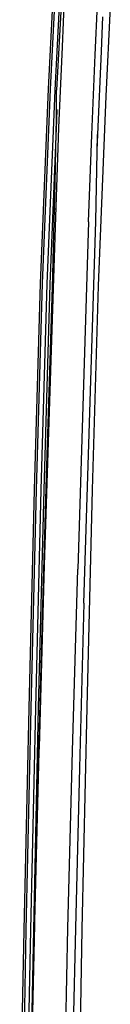
# Model space of a CAD drawing. Units: inches. Extents: x 22042254 to 25404563, y 17568978 to 17626777.
# Tile 28 of 45: x 22179871 to 22179874, y 17626261 to 17626295. Entities that reach past the tile are written whole.
import ezdxf

# ---------------------------------------------------------------- set-up
doc = ezdxf.new("R2010")
doc.units = ezdxf.units.IN
doc.header["$MEASUREMENT"] = 0
doc.layers.add('A-SITE-VEHI', color=8, linetype='Continuous', lineweight=18)
doc.layers.add('Edges', color=250, linetype='Continuous')

# ---------------------------------------------------------------- blocks, each defined once
blk = doc.blocks.new('Nissan Qashqai pl')
at = {"layer": 'Edges'}
for p, q in [((9.47817, 12.50238), (9.55025, 12.49865)), ((9.55025, 12.49865), (9.70295, 12.4926)), ((9.51676, 12.49029), (9.47609, 12.49194)), ((9.48618, 12.49606), (9.51403, 12.49492)), ((9.51403, 12.49492), (9.58109, 12.49201)), ((9.5812, 12.48741), (9.51676, 12.49029)), ((9.65101, 12.49061), (9.58109, 12.49201)), ((9.58109, 12.49201), (9.59402, 12.49144)), ((9.95835, 12.48118), (9.65101, 12.49061)), ((9.70295, 12.4926), (9.86731, 12.48784)), ((9.65144, 12.48494), (9.5812, 12.48741)), ((9.65144, 12.48494), (9.93119, 12.47609)), ((9.86731, 12.48784), (10.0423, 12.48349)), ((9.95835, 12.48118), (10.09097, 12.47751)), ((10.0423, 12.48349), (10.22109, 12.47954)), ((10.07764, 12.47192), (9.93119, 12.47609)), ((10.09097, 12.47751), (10.22022, 12.47426)), ((10.22022, 12.47426), (10.22032, 12.47426)), ((10.22032, 12.47426), (10.33528, 12.47169)), ((10.22109, 12.47954), (10.39547, 12.47621)), ((9.46937, 12.46538), (9.51052, 12.46369)), ((10.22011, 12.46826), (10.07764, 12.47192)), ((10.35861, 12.46509), (10.22011, 12.46826)), ((9.54456, 12.4542), (9.47093, 12.45809)), ((9.472, 12.46296), (9.54539, 12.4591)), ((9.47204, 12.46141), (9.54539, 12.45756)), ((9.51052, 12.46369), (9.57554, 12.46075)), ((9.54539, 12.4591), (9.54543, 12.45933)), ((9.56952, 12.45891), (9.54539, 12.4591)), ((9.54539, 12.45756), (9.70143, 12.45125)), ((9.56093, 12.45926), (9.56952, 12.45891)), ((9.57857, 12.45884), (9.56952, 12.45891)), ((9.56952, 12.45891), (9.70145, 12.45357)), ((9.57554, 12.46075), (9.64722, 12.4581)), ((9.62057, 12.45805), (9.57857, 12.45884)), ((9.67137, 12.45674), (9.62057, 12.45805)), ((9.64138, 12.45797), (9.64074, 12.45805)), ((9.64722, 12.4581), (9.92779, 12.44922)), ((9.65488, 12.4576), (9.6558, 12.45739)), ((9.47056, 12.45614), (9.54428, 12.45224)), ((9.54428, 12.45224), (9.70104, 12.44587)), ((9.70113, 12.44784), (9.54456, 12.4542)), ((9.68254, 12.4564), (9.67137, 12.45674)), ((9.68254, 12.4564), (9.68291, 12.45629)), ((9.69431, 12.45603), (9.68254, 12.4564)), ((9.69434, 12.45583), (9.69431, 12.45603)), ((9.69509, 12.45601), (9.69431, 12.45603)), ((9.69512, 12.4558), (9.69509, 12.45601)), ((9.85647, 12.45103), (9.69509, 12.45601)), ((9.70143, 12.45125), (9.86732, 12.44644)), ((9.70145, 12.45357), (9.86731, 12.44875)), ((9.97941, 12.44748), (9.85647, 12.45103)), ((9.70104, 12.44587), (9.86732, 12.44104)), ((9.86732, 12.44301), (9.70113, 12.44784)), ((9.86731, 12.44875), (10.04288, 12.4444)), ((9.86732, 12.44644), (10.04287, 12.44208)), ((10.04305, 12.43867), (9.86732, 12.44301)), ((9.92779, 12.44922), (10.07466, 12.44503)), ((10.09981, 12.44425), (9.97941, 12.44748)), ((10.04287, 12.44208), (10.22152, 12.43812)), ((10.04288, 12.4444), (10.22157, 12.44045)), ((10.07466, 12.44503), (10.07798, 12.44493)), ((10.07798, 12.44493), (10.21458, 12.44142)), ((10.21458, 12.44142), (10.09981, 12.44425)), ((9.86732, 12.44104), (10.0431, 12.4367)), ((10.22178, 12.43472), (10.04305, 12.43867)), ((10.0431, 12.4367), (10.22184, 12.43275)), ((10.21458, 12.44142), (10.21754, 12.44134)), ((10.21754, 12.44134), (10.35645, 12.43816)), ((10.22152, 12.43812), (10.39455, 12.43477)), ((10.22157, 12.44045), (10.3947, 12.43709)), ((10.39472, 12.43136), (10.22178, 12.43472)), ((10.22184, 12.43275), (10.39471, 12.42939))]:
    blk.add_line(p, q, dxfattribs=at)
blk = doc.blocks.new('CAR')
blk.add_blockref('Nissan Qashqai pl', (-9.74328, -11.91512))

msp = doc.modelspace()

# ---------------------------------------------------------------- block references
at = {"layer": 'A-SITE-VEHI', "xscale": 43.56002006885659, "yscale": 43.56002006885659, "zscale": 43.56002006885659, "rotation": 270}
msp.add_blockref('CAR', (22179848.861, 17626284.325), dxfattribs=at)

doc.saveas('drawing.dxf')
